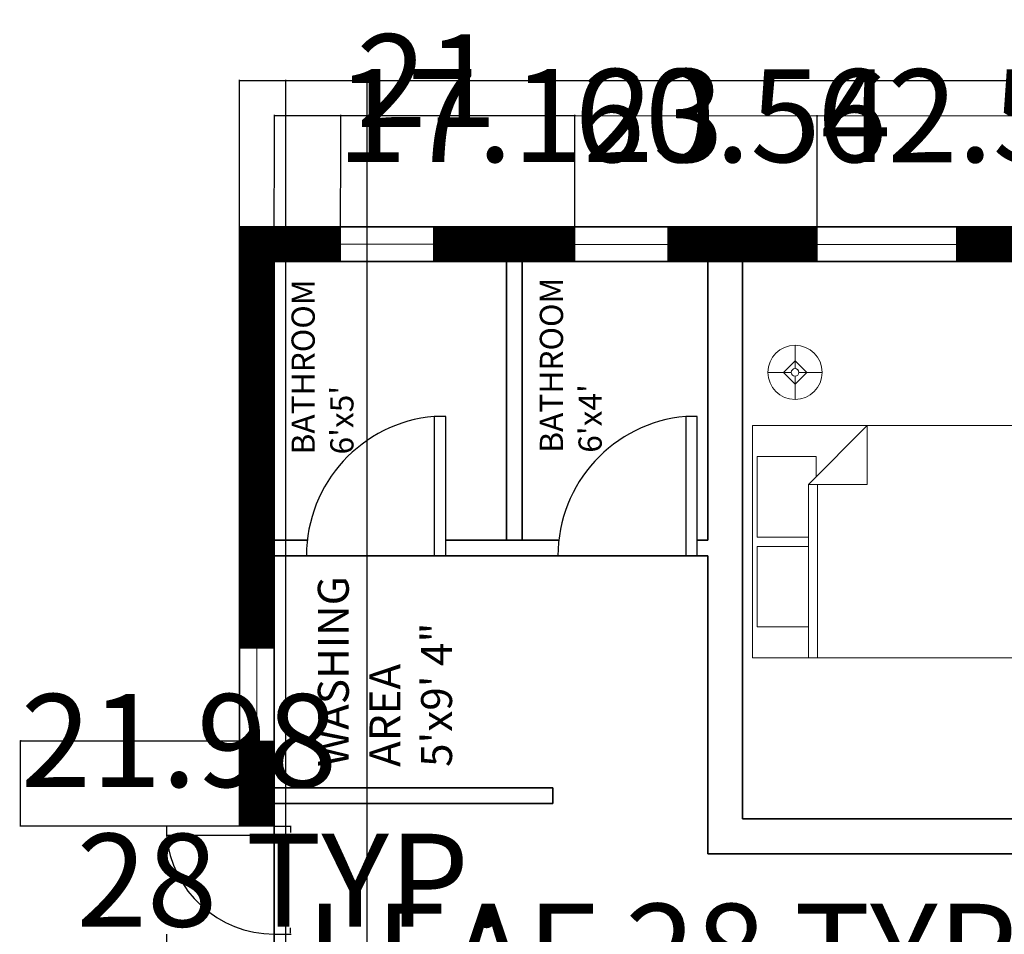
# Model space of a CAD drawing. Units: inches. Extents: x -1226 to 4538, y -998 to 1029.
# Tile 2 of 5: x -1118 to -864, y -767 to -531. Entities that reach past the tile are written whole.
import ezdxf

# ---------------------------------------------------------------- set-up
doc = ezdxf.new("R2010")
doc.units = ezdxf.units.IN
doc.header["$MEASUREMENT"] = 0
for name, color, linetype, lineweight in [('A-ANNO-DIMS', 2, 'Continuous', 18), ('A-AREA-IDEN', 7, 'Continuous', 18), ('A-DOOR', 4, 'Continuous', 25), ('A-FURN', 8, 'Continuous', 18), ('A-GLAZ', 3, 'Continuous', 18), ('A-WALL', 7, 'Continuous', 35), ('A-WALL-PATT', 1, 'Continuous', 13)]:
    doc.layers.add(name, color=color, linetype=linetype, lineweight=lineweight)
doc.styles.get("Standard").update_dxf_attribs({"font": 'arial.ttf'})
doc.dimstyles.get("Standard").update_dxf_attribs({"dimtxt": 24, "dimasz": 0.18, "dimexe": 0.18, "dimexo": 0.0625, "dimgap": 0.09, "dimtad": 0, "dimtih": 1, "dimtoh": 1, "dimdec": 0, "dimzin": 0, "dimdsep": 46, "dimlunit": 4, "dimtxsty": 'Standard', "dimcen": 0.09, "dimadec": 0, "dimazin": 0, "dimtfac": 1, "dimtdec": 0, "dimtofl": 0, "dimtmove": 0, "dimatfit": 3, "dimfxl": 1, "dimtolj": 1, "dimtzin": 0, "dimarcsym": 0})

# ---------------------------------------------------------------- blocks, each defined once
blk = doc.blocks.new('Bed - Queen')
for p, q in [((0, -80.00003), (0, 0)), ((0, 0), (59.99999, 0)), ((59.99999, 0), (59.99999, -80.00003)), ((7.99999, -1.2), (28.79998, -1.2)), ((7.99999, -14.4), (7.99999, -1.2)), ((28.79998, -1.2), (28.79998, -14.4)), ((31.19999, -1.2), (51.99999, -1.2)), ((31.19999, -14.4), (31.19999, -1.2)), ((51.99999, -1.2), (51.99999, -16.4)), ((0, -14.4), (44.8, -14.4)), ((59.99999, -29.6), (44.8, -14.4)), ((44.8, -14.4), (44.8, -29.6)), ((44.8, -16.8), (0, -16.8)), ((51.99999, -16.4), (46.79936, -16.4)), ((44.8, -29.6), (59.99999, -29.6)), ((59.99999, -80.00003), (0, -80.00003))]:
    blk.add_line(p, q)
blk = doc.blocks.new('Lamp - Table')
for p, q in [((0, 7), (0, 1)), ((0, 3), (-3, 0)), ((3, 0), (0, 3)), ((-1, 0), (-7, 0)), ((-3, 0), (0, -3)), ((0, -3), (3, 0)), ((1, 0), (7, 0)), ((0, -1), (0, -7))]:
    blk.add_line(p, q)
for radius in [7, 1]:
    blk.add_circle((0, 0), radius)
blk = doc.blocks.new('DOOR-SWING-36')
for p, q in [((36, 36), (0, 36)), ((0, 36), (0, 33)), ((36, 33), (36, 36)), ((0, 33), (36, 33))]:
    blk.add_line(p, q)
blk.add_arc((36, 36.14), 36.14, 184.9791, 270)
blk = doc.blocks.new('DOOR-SWING-NARROW')
for p, q in [((27.84, 27.84), (0, 27.84)), ((0, 27.84), (0, 25.52)), ((0, 25.52), (27.84, 25.52)), ((27.84, 25.52), (27.84, 27.84))]:
    blk.add_line(p, q)
blk.add_arc((27.84, 27.94), 27.94, 184.9791, 270)
blk = doc.blocks.new('WIN-36')
for p, q in [((0, 36), (9, 36)), ((4.5, 0), (4.5, 36)), ((0, 0), (9, 0))]:
    blk.add_line(p, q)
blk = doc.blocks.new('WIN-24')
for p, q in [((0, 24), (9, 24)), ((4.5, 0), (4.5, 24)), ((0, 0), (9, 0))]:
    blk.add_line(p, q)
blk = doc.blocks.new('*D28')
at = {"layer": 'A-ANNO-DIMS', "color": 0, "lineweight": -2, "transparency": 16777216}
for p, q in [((-1080.03, -767.33), (-1080.03, -771.62)), ((-1052.19, -767.33), (-1052.19, -771.62)), ((-1079.85, -771.44), (-1052.37, -771.44)), ((-1052.19, -771.44), (-1052.01, -771.44))]:
    blk.add_line(p, q, dxfattribs=at)
at = {"layer": 'A-ANNO-DIMS', "color": 0, "transparency": 16777216}
for points in [[(-1079.85, -771.41), (-1079.85, -771.47), (-1080.03, -771.44)], [(-1052.37, -771.41), (-1052.37, -771.47), (-1052.19, -771.44)]]:
    blk.add_solid(points, dxfattribs=at)
at = {"layer": 'Defpoints', "color": 0, "transparency": 16777216}
for p in [(-1080.03, -767.26), (-1052.19, -767.26), (-1052.19, -771.44)]:
    blk.add_point(p, dxfattribs=at)
at = {"layer": 'A-ANNO-DIMS', "color": 0, "transparency": 16777216, "insert": (-947.45, -771.44), "char_height": 24, "attachment_point": 5}
blk.add_mtext('\\A1;LEAF 28 TYP.', dxfattribs=at)
blk = doc.blocks.new('*D29')
at = {"layer": 'A-ANNO-DIMS', "color": 0, "lineweight": -2, "transparency": 16777216}
for p, q in [((-1052.13, -739.42), (-1047.83, -739.42)), ((-1048.01, -739.6), (-1048.01, -741)), ((-1048.01, -767.08), (-1048.01, -765.69)), ((-1052.13, -767.26), (-1047.83, -767.26))]:
    blk.add_line(p, q, dxfattribs=at)
at = {"layer": 'A-ANNO-DIMS', "color": 0, "transparency": 16777216}
for points in [[(-1048.04, -739.6), (-1047.98, -739.6), (-1048.01, -739.42)], [(-1048.04, -767.08), (-1047.98, -767.08), (-1048.01, -767.26)]]:
    blk.add_solid(points, dxfattribs=at)
at = {"layer": 'Defpoints', "color": 0, "transparency": 16777216}
for p in [(-1052.19, -739.42), (-1048.01, -739.42), (-1052.19, -767.26)]:
    blk.add_point(p, dxfattribs=at)
at = {"layer": 'A-ANNO-DIMS', "color": 0, "transparency": 16777216, "insert": (-1048.01, -753.34), "char_height": 24, "attachment_point": 5}
blk.add_mtext('\\A1;28 TYP.', dxfattribs=at)
blk = doc.blocks.new('*D48')
at = {"layer": 'A-ANNO-DIMS', "color": 0, "lineweight": -2, "transparency": 16777216}
for p, q in [((-1061.17, -584.46), (-1061.17, -546.6)), ((-1060.99, -546.78), (-776.71, -546.78)), ((-439.35, -546.78), (-723.62, -546.78)), ((-439.17, -584.46), (-439.17, -546.6))]:
    blk.add_line(p, q, dxfattribs=at)
at = {"layer": 'A-ANNO-DIMS', "color": 0, "transparency": 16777216}
for points in [[(-1060.99, -546.75), (-1060.99, -546.81), (-1061.17, -546.78)], [(-439.35, -546.75), (-439.35, -546.81), (-439.17, -546.78)]]:
    blk.add_solid(points, dxfattribs=at)
at = {"layer": 'Defpoints', "color": 0, "transparency": 16777216}
for p in [(-439.17, -546.78), (-1061.17, -584.53), (-439.17, -584.53)]:
    blk.add_point(p, dxfattribs=at)
at = {"layer": 'A-ANNO-DIMS', "color": 0, "transparency": 16777216, "insert": (-750.17, -546.78), "char_height": 24, "attachment_point": 5}
blk.add_mtext('\\A1;622', dxfattribs=at)
blk = doc.blocks.new('*D50')
at = {"layer": 'A-ANNO-DIMS', "color": 0, "lineweight": -2, "transparency": 16777216}
for p, q in [((-1052.17, -593.46), (-1052.14, -555.6)), ((-1051.96, -555.78), (-1035.2, -555.79)), ((-1035.04, -593.48), (-1035.02, -555.61)), ((-1035.02, -555.79), (-1034.84, -555.79))]:
    blk.add_line(p, q, dxfattribs=at)
at = {"layer": 'A-ANNO-DIMS', "color": 0, "transparency": 16777216}
for points in [[(-1051.96, -555.75), (-1051.96, -555.81), (-1052.14, -555.78)], [(-1035.2, -555.76), (-1035.2, -555.82), (-1035.02, -555.79)]]:
    blk.add_solid(points, dxfattribs=at)
at = {"layer": 'Defpoints', "color": 0, "transparency": 16777216}
for p in [(-1035.02, -555.79), (-1052.17, -593.53), (-1035.04, -593.54)]:
    blk.add_point(p, dxfattribs=at)
at = {"layer": 'A-ANNO-DIMS', "color": 0, "transparency": 16777216, "insert": (-986.06, -555.79), "char_height": 24, "attachment_point": 5}
blk.add_mtext('\\A1;17.123', dxfattribs=at)
blk = doc.blocks.new('*D51')
at = {"layer": 'A-ANNO-DIMS', "color": 0, "lineweight": -2, "transparency": 16777216}
for p, q in [((-1035.04, -593.48), (-1035.02, -555.61)), ((-1034.84, -555.79), (-974.67, -555.82)), ((-974.51, -593.51), (-974.49, -555.64)), ((-974.49, -555.82), (-974.31, -555.82))]:
    blk.add_line(p, q, dxfattribs=at)
at = {"layer": 'A-ANNO-DIMS', "color": 0, "transparency": 16777216}
for points in [[(-1034.84, -555.76), (-1034.84, -555.82), (-1035.02, -555.79)], [(-974.67, -555.79), (-974.67, -555.85), (-974.49, -555.82)]]:
    blk.add_solid(points, dxfattribs=at)
at = {"layer": 'Defpoints', "color": 0, "transparency": 16777216}
for p in [(-974.49, -555.82), (-1035.04, -593.54), (-974.51, -593.57)]:
    blk.add_point(p, dxfattribs=at)
at = {"layer": 'A-ANNO-DIMS', "color": 0, "transparency": 16777216, "insert": (-933.71, -555.82), "char_height": 24, "attachment_point": 5}
blk.add_mtext('\\A1;60.54', dxfattribs=at)
blk = doc.blocks.new('*D52')
at = {"layer": 'A-ANNO-DIMS', "color": 0, "lineweight": -2, "transparency": 16777216}
for p, q in [((-974.51, -593.51), (-974.49, -555.64)), ((-974.31, -555.82), (-912.1, -555.84)), ((-911.93, -593.53), (-911.92, -555.66)), ((-911.92, -555.84), (-911.74, -555.84))]:
    blk.add_line(p, q, dxfattribs=at)
at = {"layer": 'A-ANNO-DIMS', "color": 0, "transparency": 16777216}
for points in [[(-974.31, -555.79), (-974.31, -555.85), (-974.49, -555.82)], [(-912.1, -555.81), (-912.1, -555.87), (-911.92, -555.84)]]:
    blk.add_solid(points, dxfattribs=at)
at = {"layer": 'Defpoints', "color": 0, "transparency": 16777216}
for p in [(-911.92, -555.84), (-974.51, -593.57), (-911.93, -593.59)]:
    blk.add_point(p, dxfattribs=at)
at = {"layer": 'A-ANNO-DIMS', "color": 0, "transparency": 16777216, "insert": (-871.06, -555.84), "char_height": 24, "attachment_point": 5}
blk.add_mtext('\\A1;62.58', dxfattribs=at)
blk = doc.blocks.new('*D53')
at = {"layer": 'A-ANNO-DIMS', "color": 0, "lineweight": -2, "transparency": 16777216}
for p, q in [((-911.93, -593.53), (-911.94, -555.66)), ((-911.76, -555.84), (-850, -555.82)), ((-737.11, -555.8), (-798.87, -555.81)), ((-736.92, -593.48), (-736.93, -555.62))]:
    blk.add_line(p, q, dxfattribs=at)
at = {"layer": 'A-ANNO-DIMS', "color": 0, "transparency": 16777216}
for points in [[(-911.76, -555.81), (-911.76, -555.87), (-911.94, -555.84)], [(-737.11, -555.77), (-737.11, -555.83), (-736.93, -555.8)]]:
    blk.add_solid(points, dxfattribs=at)
at = {"layer": 'Defpoints', "color": 0, "transparency": 16777216}
for p in [(-736.93, -555.8), (-911.93, -593.59), (-736.92, -593.55)]:
    blk.add_point(p, dxfattribs=at)
at = {"layer": 'A-ANNO-DIMS', "color": 0, "transparency": 16777216, "insert": (-824.43, -555.82), "char_height": 24, "attachment_point": 5}
blk.add_mtext('\\A1;175', dxfattribs=at)
blk = doc.blocks.new('*D61')
at = {"layer": 'A-ANNO-DIMS', "color": 0, "lineweight": -2, "transparency": 16777216}
for p, q in [((-1117.78, -717.45), (-1117.78, -717.27)), ((-1117.78, -717.27), (-1117.6, -717.27)), ((-1061.24, -717.45), (-1117.96, -717.45)), ((-1117.78, -739.24), (-1117.78, -717.63)), ((-1061.23, -739.42), (-1117.96, -739.42))]:
    blk.add_line(p, q, dxfattribs=at)
at = {"layer": 'A-ANNO-DIMS', "color": 0, "transparency": 16777216}
for points in [[(-1117.81, -717.63), (-1117.75, -717.63), (-1117.78, -717.45)], [(-1117.81, -739.24), (-1117.75, -739.24), (-1117.78, -739.42)]]:
    blk.add_solid(points, dxfattribs=at)
at = {"layer": 'Defpoints', "color": 0, "transparency": 16777216}
for p in [(-1117.78, -717.45), (-1061.18, -717.45), (-1061.17, -739.42)]:
    blk.add_point(p, dxfattribs=at)
at = {"layer": 'A-ANNO-DIMS', "color": 0, "transparency": 16777216, "insert": (-1076.78, -717.27), "char_height": 24, "attachment_point": 5}
blk.add_mtext('\\A1;21.98', dxfattribs=at)
blk = doc.blocks.new('*D77')
at = {"layer": 'A-ANNO-DIMS', "color": 0, "lineweight": -2, "transparency": 16777216}
for p, q in [((-1049.16, -851.5), (-1049.16, -546.6)), ((-1048.98, -546.78), (-1028.34, -546.78)), ((-1028.16, -851.5), (-1028.16, -546.6)), ((-1028.16, -546.78), (-1027.98, -546.78))]:
    blk.add_line(p, q, dxfattribs=at)
at = {"layer": 'A-ANNO-DIMS', "color": 0, "transparency": 16777216}
for points in [[(-1048.98, -546.75), (-1048.98, -546.81), (-1049.16, -546.78)], [(-1028.34, -546.75), (-1028.34, -546.81), (-1028.16, -546.78)]]:
    blk.add_solid(points, dxfattribs=at)
at = {"layer": 'Defpoints', "color": 0, "transparency": 16777216}
for p in [(-1028.16, -546.78), (-1049.16, -851.56), (-1028.16, -851.56)]:
    blk.add_point(p, dxfattribs=at)
at = {"layer": 'A-ANNO-DIMS', "color": 0, "transparency": 16777216, "insert": (-1012.81, -546.78), "char_height": 24, "attachment_point": 5}
blk.add_mtext('\\A1;21', dxfattribs=at)

msp = doc.modelspace()

# ---------------------------------------------------------------- hatches: boundary and pattern name
at = {"layer": 'A-WALL-PATT'}
h = msp.add_hatch(dxfattribs=at)
h.set_pattern_fill('ANSI31', color=256, angle=90)
h.set_pattern_definition([(135, (-1048.80633, 527.86775), (-0.088388348, -0.088388348), [])])
h.paths.add_polyline_path([(-1052.1662, -935.5274), (-1052.1662, -878.4295), (-1061.1662, -878.4295), (-1061.1662, -944.5274), (-1012.2132, -944.5274), (-1012.2132, -935.5274)])
h.paths.add_polyline_path([(-976.2132, -935.5274), (-976.2132, -944.5274), (-730.4734, -944.5274), (-730.4734, -935.5274)])
h.paths.add_polyline_path([(-694.4734, -935.5274), (-694.4734, -944.5274), (-651.0832, -944.5274), (-651.0832, -935.5274)])
h.paths.add_polyline_path([(-615.0832, -935.5274), (-615.0832, -944.5274), (-561.1662, -944.5274), (-561.1662, -935.5274)])
h.paths.add_polyline_path([(-712.9165, -584.5274), (-712.9165, -593.5274), (-657.3138, -593.5274), (-657.3138, -593.4838), (-597.3139, -593.4838), (-448.1662, -593.5274), (-448.1662, -713.5274), (-448.1662, -779.5274), (-439.1662, -779.5274), (-439.1662, -584.5274)])
h.paths.add_polyline_path([(-875.9292, -584.5274), (-875.9292, -593.5274), (-736.9165, -593.5274), (-736.9165, -584.5274)])
h.paths.add_polyline_path([(-950.5052, -584.5274), (-950.5052, -593.5274), (-911.9292, -593.5274), (-911.9292, -584.5274)])
h.paths.add_polyline_path([(-1011.0429, -584.5274), (-1011.0429, -593.5274), (-974.5052, -593.5274), (-974.5052, -584.5274)])
h.paths.add_polyline_path([(-1061.1662, -584.5274), (-1061.1662, -693.4459), (-1052.1662, -693.4459), (-1052.1662, -593.5274), (-1035.0429, -593.5274), (-1035.0429, -584.5274)])
h.paths.add_polyline_path([(-1061.1662, -795.2404), (-1061.1662, -842.4295), (-1052.1662, -842.4295), (-1052.1662, -795.2404)])
h.paths.add_polyline_path([(-1061.1662, -717.4459), (-1061.1662, -739.4249), (-1052.1662, -739.4249), (-1052.1662, -717.4459)])

# ---------------------------------------------------------------- linework, layer by layer
at = {"layer": 'A-WALL'}
for p, q in [((-1061.1662, -584.5274), (-439.1662, -584.5274)), ((-1061.1662, -739.4249), (-1061.1662, -584.5274)), ((-1052.1662, -935.5274), (-1052.1662, -593.5274)), ((-1052.1662, -593.5274), (-448.1662, -593.5274)), ((-992.1662, -665.5274), (-992.1662, -593.5274)), ((-988.1662, -665.5274), (-988.1662, -593.5274)), ((-940.1662, -665.5274), (-940.1662, -593.5274)), ((-931.1662, -737.5274), (-931.1662, -593.5274)), ((-1052.1662, -665.5274), (-1043.6444, -665.5274)), ((-1007.8659, -665.5274), (-978.6599, -665.5274)), ((-942.8833, -665.5274), (-940.1662, -665.5274)), ((-1052.1662, -669.5274), (-940.1662, -669.5274)), ((-940.1662, -746.5274), (-940.1662, -669.5274)), ((-1052.1662, -729.5274), (-980.1662, -729.5274)), ((-980.1662, -733.5274), (-980.1662, -729.5274)), ((-1052.1662, -733.5274), (-980.1662, -733.5274)), ((-931.1662, -737.5274), (-835.06, -737.5274)), ((-940.1662, -746.5274), (-836.2644, -746.5274))]:
    msp.add_line(p, q, dxfattribs=at)

# ---------------------------------------------------------------- block references
at = {"layer": 'A-DOOR'}
for p, rotation in [((-1043.8661, -633.5233), 270.0000000000001), ((-978.8835, -633.5399), 269.9999999999998)]:
    msp.add_blockref('DOOR-SWING-36', p, dxfattribs=dict(at, rotation=rotation))
msp.add_blockref('DOOR-SWING-NARROW', (-1080.027, -767.264), dxfattribs=at)
at = {"layer": 'A-FURN', "rotation": 90}
for name, p in [('Lamp - Table', (-917.612, -622.1588)), ('Bed - Queen', (-928.5798, -695.9107))]:
    msp.add_blockref(name, p, dxfattribs=at)
at = {"layer": 'A-GLAZ'}
for name, p, rotation in [('WIN-24', (-1035.043, -584.5398), 269.9999999999983), ('WIN-24', (-974.5053, -584.5693), 269.9999999999977), ('WIN-36', (-911.9287, -584.5893), 270.0000000000006)]:
    msp.add_blockref(name, p, dxfattribs=dict(at, rotation=rotation))
msp.add_blockref('WIN-24', (-1061.177, -717.446), dxfattribs=at)

# ---------------------------------------------------------------- texts
at = {"layer": 'A-AREA-IDEN', "attachment_point": 1, "rotation": 90}
for s, width, heights, insert, char_height in [("BATHROOM\\P6'x5'", 30.339854, [19.7709], (-1047.719, -643.3543), 6), ("BATHROOM\\P6'x4'", 30.339854, [19.7709], (-983.5733, -642.9146), 6), ('WASHING AREA\\P5\'x9\' 4"', 40.89133, [0], (-1040.9241, -724.0867), 8)]:
    msp.add_mtext_dynamic_manual_height_columns(s, width=width, gutter_width=1, heights=heights, dxfattribs=dict(at, insert=insert, char_height=char_height))

# ---------------------------------------------------------------- dimensions: what is measured, and where the dimension line sits
at = {"layer": 'A-ANNO-DIMS'}
for base, p1, p2, picture, middle in [((-439.1662, -546.7774), (-1061.1662, -584.5274), (-439.1662, -584.5274), '*D48', (-750.1662, -546.7774)), ((-1028.1562, -546.7774), (-1049.1562, -851.5639), (-1028.1562, -851.5639), '*D77', (-1012.8084, -546.7774))]:
    dim = msp.add_linear_dim(base=base, p1=p1, p2=p2, dimstyle='Standard', override={"dimdec": 0, "dimlfac": 1, "dimrnd": 0, "dimzin": 0, "dimdsep": 46, "dimlunit": 2}, dxfattribs=at)
    dim.commit()
    dim.dimension.update_dxf_attribs({"geometry": picture, "text_midpoint": middle})
for base, p1, p2, angle, override, picture, middle in [((-1035.0164, -555.7895), (-1052.1662, -593.5274), (-1035.0429, -593.5395), 359.959736, {"dimdec": 3, "dimlfac": 1, "dimrnd": 0, "dimzin": 0, "dimdsep": 46, "dimlunit": 2}, '*D50', (-986.0588, -555.7896)), ((-974.4868, -555.819), (-1035.0429, -593.5395), (-974.5052, -593.569), 359.972083, {"dimdec": 2, "dimlfac": 1, "dimrnd": 0, "dimzin": 0, "dimdsep": 46, "dimlunit": 2}, '*D51', (-933.7066, -555.8191)), ((-911.9169, -555.8393), (-974.5052, -593.569), (-911.9292, -593.5893), 359.981403, {"dimdec": 2, "dimlfac": 1, "dimrnd": 0, "dimzin": 0, "dimdsep": 46, "dimlunit": 2}, '*D52', (-871.063, -555.8393)), ((-736.9259, -555.7956), (-911.9292, -593.5893), (-736.9165, -593.5456), 0.014311, {"dimdec": 0, "dimlfac": 1, "dimrnd": 0, "dimzin": 0, "dimdsep": 46, "dimlunit": 2}, '*D53', (-824.4323, -555.8174)), ((-1117.7772, -717.4459), (-1061.1662, -739.4249), (-1061.1773, -717.4459), 90, {"dimdec": 2, "dimlfac": 1, "dimrnd": 0, "dimzin": 0, "dimdsep": 46, "dimlunit": 2}, '*D61', (-1076.7841, -717.2659))]:
    dim = msp.add_linear_dim(base=base, p1=p1, p2=p2, angle=angle, dimstyle='Standard', override=override, dxfattribs=at)
    dim.commit()
    dim.dimension.update_dxf_attribs({"geometry": picture, "text_midpoint": middle})
dim = msp.add_linear_dim(base=(-1052.1878, -771.4403), p1=(-1080.0272, -767.2643), p2=(-1052.1878, -767.2643), text='LEAF <> TYP.', dimstyle='Standard', override={"dimdec": 0, "dimlfac": 1, "dimrnd": 0, "dimzin": 0, "dimdsep": 46, "dimlunit": 2}, dxfattribs=at)
dim.commit()
dim.dimension.update_dxf_attribs({"geometry": '*D28', "text_midpoint": (-947.4539, -771.4403)})
dim = msp.add_linear_dim(base=(-1048.0119, -739.4249), p1=(-1052.1878, -767.2643), p2=(-1052.1878, -739.4249), angle=90, text='<> TYP.', dimstyle='Standard', override={"dimdec": 0, "dimlfac": 1, "dimrnd": 0, "dimzin": 0, "dimdsep": 46, "dimlunit": 2}, dxfattribs=at)
dim.commit()
dim.dimension.update_dxf_attribs({"geometry": '*D29', "text_midpoint": (-1048.0119, -753.3446)})

doc.saveas('drawing.dxf')
